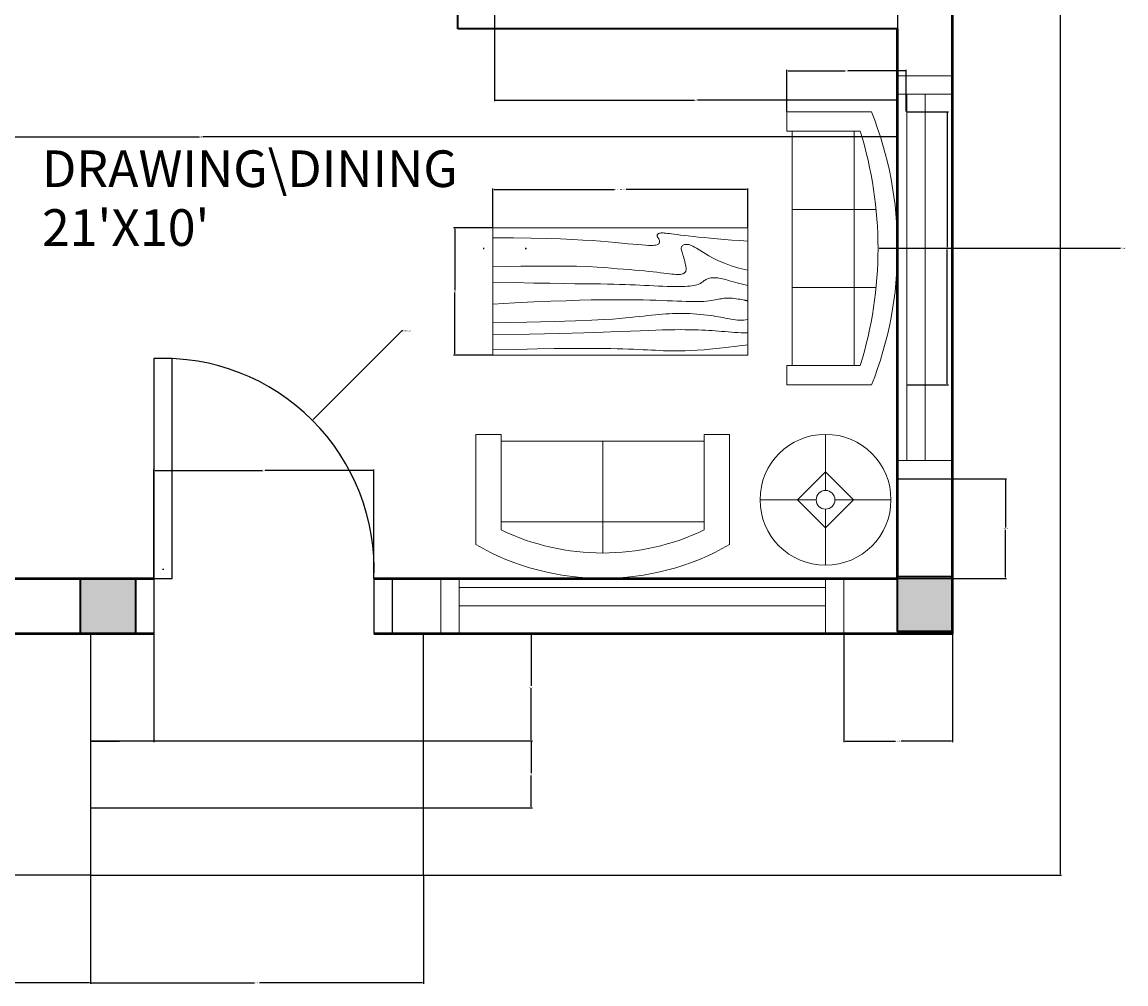
# Model space of a CAD drawing. Units: inches. Extents: x 2421 to 2780, y 382 to 769.
# Tile 2 of 4: x 2599 to 2780, y 382 to 539. Entities that reach past the tile are written whole.
import ezdxf

# ---------------------------------------------------------------- set-up
doc = ezdxf.new("R2010")
doc.units = ezdxf.units.IN
for name, color, linetype, lineweight in [('A-ANNO-DIMS', 2, 'Continuous', 18), ('A-AREA-IDEN', 7, 'Continuous', 25), ('A-COLS', 1, 'Continuous', 35), ('A-FLOR-STRS', 7, 'Continuous', 25), ('DOOR', 1, 'Continuous', 25), ('FURNITURE', 3, 'Continuous', 18), ('INNER WALL', 2, 'Continuous', 35), ('OUTER WALL', 4, 'Continuous', 50), ('WINDOW', 5, 'Continuous', 18)]:
    doc.layers.add(name, color=color, linetype=linetype, lineweight=lineweight)
doc.styles.get("Standard").update_dxf_attribs({"font": 'arial.ttf'})
doc.dimstyles.get("Standard").update_dxf_attribs({"dimtxt": 0.18, "dimasz": 0.18, "dimexe": 0.18, "dimexo": 0.0625, "dimgap": 0.09, "dimtad": 0, "dimtih": 1, "dimtoh": 1, "dimdec": 4, "dimzin": 0, "dimdsep": 46, "dimtxsty": 'Standard', "dimcen": 0.09, "dimadec": 0, "dimazin": 0, "dimtfac": 1, "dimtdec": 4, "dimtofl": 0, "dimtmove": 0, "dimatfit": 3, "dimfxl": 1, "dimtolj": 1, "dimtzin": 0, "dimarcsym": 0})

# ---------------------------------------------------------------- blocks, each defined once
blk = doc.blocks.new('Sofa - Roundback 7 ft.')
for p, q in [((-12.00002, -32.4421), (-12.00003, -6.5971)), ((11.99997, -32.4421), (11.99998, -6.5971)), ((-36.000027, -34), (-36.000027, -11.4696)), ((-35.999844, -13.3819), (35.9998, -13.3819)), ((35.99998, -34), (35.99998, -11.4696)), ((-36.000027, -32.4421), (35.99998, -32.4421))]:
    blk.add_line(p, q)
for points in [[(-36.000027, -34), (-42.000027, -34), (-42.000027, -8)], [(41.99998, -8), (41.99998, -34), (35.99998, -34)]]:
    blk.add_lwpolyline(points)
for centre, radius, start, end in [((0, -114.25), 114.25, 68.43141, 111.5686), ((-0.00001, -127.1968), 121.1968, 72.72033, 107.2797)]:
    blk.add_arc(centre, radius, start, end)
blk = doc.blocks.new('Table - Rectangular Woodgrain 60 x 30 in.')
for p, q in [((0, 0), (0, -30)), ((60, 0), (0, 0)), ((60, -30), (60, 0)), ((0, -30), (60, -30))]:
    blk.add_line(p, q)
for points in [[(0, -2.4), (4.8155, -2.418), (9.0302, -2.4688), (12.709, -2.5477), (15.9167, -2.65), (18.7181, -2.7711), (21.1781, -2.9063), (23.3616, -3.0508), (25.3333, -3.2), (27.1477, -3.3495), (28.8172, -3.4958), (30.3437, -3.636), (31.7291, -3.7667), (32.9756, -3.8849), (34.0849, -3.9875), (35.059, -4.0714), (35.9, -4.1334), (36.6114, -4.1711), (37.2041, -4.1854), (37.6906, -4.1779), (38.0833, -4.15), (38.3948, -4.1034), (38.6375, -4.0396), (38.8239, -3.9602), (38.9666, -3.8667), (39.0764, -3.7608), (39.1573, -3.6448), (39.2116, -3.521), (39.2416, -3.3917), (39.2498, -3.2593), (39.2385, -3.1261), (39.21, -2.9944), (39.1666, -2.8667), (39.111, -2.7447), (39.0468, -2.6281), (38.978, -2.5163), (38.9083, -2.4083), (38.8418, -2.3035), (38.7823, -2.201), (38.7337, -2.1001), (38.7, -2), (38.6844, -1.9003), (38.6875, -1.8021), (38.7094, -1.707), (38.75, -1.6167), (38.8094, -1.5326), (38.8875, -1.4563), (38.9844, -1.3893), (39.1, -1.3333), (39.2351, -1.2896), (39.3937, -1.2583), (39.5804, -1.2396), (39.8, -1.2333), (40.057, -1.2396), (40.3562, -1.2583), (40.7023, -1.2896), (41.1, -1.3333), (41.5547, -1.3895), (42.0755, -1.4573), (42.6721, -1.5361), (43.3542, -1.625), (44.1316, -1.7233), (45.014, -1.8302), (46.0114, -1.9449), (47.1333, -2.0667), (48.3862, -2.1947), (49.7625, -2.3281), (51.2513, -2.4663), (52.8416, -2.6083), (54.5226, -2.7535), (56.2833, -2.9011), (58.1127, -3.0501), (60, -3.2)], [(0, -9.2), (6.5759, -9.0858), (11.9385, -9.0365), (16.2527, -9.0418), (19.6833, -9.0917), (22.3952, -9.1759), (24.5531, -9.2844), (26.322, -9.4069), (27.8666, -9.5333), (29.3241, -9.6553), (30.7203, -9.7719), (32.0532, -9.8837), (33.3208, -9.9917), (34.5213, -10.0965), (35.6526, -10.199), (36.7128, -10.2999), (37.7, -10.4), (38.6129, -10.4996), (39.4531, -10.5969), (40.223, -10.6895), (40.925, -10.775), (41.5613, -10.8512), (42.1344, -10.9156), (42.6465, -10.966), (43.1, -11), (43.4976, -11.0158), (43.8437, -11.0136), (44.143, -10.9942), (44.4, -10.9583), (44.6195, -10.9069), (44.8062, -10.8406), (44.9648, -10.7603), (45.1, -10.6667), (45.2155, -10.5598), (45.3114, -10.4365), (45.3871, -10.2929), (45.4416, -10.125), (45.4743, -9.929), (45.4844, -9.7011), (45.4709, -9.4371), (45.4333, -9.1333), (45.3716, -8.7883), (45.2896, -8.4104), (45.1919, -8.0107), (45.0833, -7.6), (44.9685, -7.1893), (44.8521, -6.7896), (44.7388, -6.4117), (44.6333, -6.0667), (44.54, -5.7628), (44.4614, -5.4979), (44.4001, -5.2675), (44.3583, -5.0667), (44.3384, -4.8909), (44.3427, -4.7354), (44.3736, -4.5956), (44.4333, -4.4667), (44.5236, -4.3453), (44.6427, -4.2333), (44.7884, -4.1339), (44.9583, -4.05), (45.1501, -3.9849), (45.3614, -3.9417), (45.59, -3.9234), (45.8333, -3.9333), (46.0915, -3.9749), (46.3734, -4.0531), (46.6906, -4.1736), (47.0542, -4.3417), (47.4756, -4.5629), (47.9661, -4.8427), (48.5372, -5.1866), (49.2, -5.6), (49.9676, -6.0844), (50.8594, -6.625), (51.8965, -7.2031), (53.1, -7.8), (54.491, -8.3969), (56.0906, -8.975), (57.9199, -9.5156), (60, -10)], [(0, -12.8), (5.1847, -12.9322), (9.6213, -13.0323), (13.3963, -13.1059), (16.5958, -13.1583), (19.3063, -13.1952), (21.614, -13.2219), (23.6054, -13.2439), (25.3666, -13.2667), (26.9728, -13.2947), (28.4531, -13.3281), (29.8256, -13.3663), (31.1083, -13.4083), (32.3191, -13.4535), (33.476, -13.501), (34.597, -13.5501), (35.7, -13.6), (36.7984, -13.6497), (37.8875, -13.6979), (38.9578, -13.743), (40, -13.7833), (41.0047, -13.8174), (41.9625, -13.8438), (42.864, -13.8607), (43.7, -13.8667), (44.4631, -13.8604), (45.1552, -13.8417), (45.7801, -13.8104), (46.3416, -13.7667), (46.8439, -13.7104), (47.2906, -13.6417), (47.6858, -13.5604), (48.0333, -13.4667), (48.3375, -13.3608), (48.6042, -13.2448), (48.8396, -13.121), (49.05, -12.9917), (49.2417, -12.8593), (49.4208, -12.7261), (49.5937, -12.5944), (49.7667, -12.4667), (49.9452, -12.3451), (50.1323, -12.2313), (50.3303, -12.1268), (50.5416, -12.0333), (50.7686, -11.9524), (51.0135, -11.8854), (51.2788, -11.8341), (51.5666, -11.8), (51.8785, -11.7843), (52.2116, -11.7865), (52.562, -11.8059), (52.926, -11.8417), (53.2998, -11.8931), (53.6795, -11.9594), (54.0614, -12.0397), (54.4416, -12.1333), (54.8223, -12.2401), (55.2293, -12.3625), (55.6942, -12.5037), (56.2489, -12.6667), (56.9251, -12.8547), (57.7545, -13.0708), (58.7689, -13.3182), (60, -13.6)], [(0, -18), (5.124, -17.7273), (9.6609, -17.5057), (13.6705, -17.3303), (17.2125, -17.1958), (20.3467, -17.0973), (23.1328, -17.0297), (25.6307, -16.9878), (27.9, -16.9667), (29.9928, -16.9617), (31.9302, -16.9703), (33.7254, -16.9907), (35.3917, -17.0208), (36.9423, -17.0588), (38.3906, -17.1026), (39.7499, -17.1503), (41.0333, -17.2), (42.2519, -17.2496), (43.4073, -17.2969), (44.4986, -17.3395), (45.525, -17.375), (46.4858, -17.4012), (47.3802, -17.4156), (48.2074, -17.416), (48.9667, -17.4), (49.6583, -17.3662), (50.2872, -17.3167), (50.8595, -17.2547), (51.3812, -17.1833), (51.8584, -17.1057), (52.2971, -17.025), (52.7034, -16.9443), (53.0833, -16.8667), (53.443, -16.7951), (53.789, -16.7313), (54.128, -16.6768), (54.4666, -16.6334), (54.8115, -16.6024), (55.1693, -16.5854), (55.5465, -16.5841), (55.95, -16.6), (56.3828, -16.6337), (56.8346, -16.6823), (57.2915, -16.7418), (57.7396, -16.8084), (58.165, -16.878), (58.5539, -16.9469), (58.8924, -17.0111), (59.1666, -17.0667), (59.3679, -17.1107), (59.5078, -17.1438), (59.6032, -17.1675), (59.6708, -17.1833), (59.7275, -17.193), (59.7901, -17.1979), (59.8753, -17.1998), (60, -17.2)], [(0, -22.4), (8.0098, -22.2501), (14.4094, -22.1011), (19.4168, -21.9535), (23.25, -21.8083), (26.1269, -21.6663), (28.2656, -21.5281), (29.884, -21.3947), (31.2, -21.2667), (32.3967, -21.1448), (33.5172, -21.0292), (34.5697, -20.9198), (35.5625, -20.8167), (36.5037, -20.7198), (37.4015, -20.6292), (38.2642, -20.5448), (39.1, -20.4667), (39.9164, -20.3951), (40.7187, -20.3313), (41.5117, -20.2768), (42.3, -20.2333), (43.0883, -20.2024), (43.8812, -20.1854), (44.6836, -20.1841), (45.5, -20.2), (46.3328, -20.234), (47.1747, -20.2844), (48.0163, -20.3488), (48.8479, -20.425), (49.66, -20.5106), (50.4429, -20.6031), (51.1872, -20.7004), (51.8833, -20.8), (52.5246, -20.8999), (53.1166, -20.9995), (53.6681, -21.0983), (54.1875, -21.1958), (54.6834, -21.2919), (55.1646, -21.3859), (55.6394, -21.4777), (56.1167, -21.5667), (56.6028, -21.6515), (57.0961, -21.7266), (57.5929, -21.7852), (58.0896, -21.8208), (58.5823, -21.8268), (59.0674, -21.7964), (59.5412, -21.723), (60, -21.6)], [(0, -25.2), (8.6355, -25.0504), (15.7026, -24.9031), (21.4049, -24.7606), (25.9458, -24.625), (29.529, -24.4988), (32.3578, -24.3844), (34.6359, -24.284), (36.5667, -24.2), (38.3213, -24.1341), (39.9417, -24.0854), (41.437, -24.0523), (42.8167, -24.0333), (44.0901, -24.0268), (45.2667, -24.0313), (46.3557, -24.0451), (47.3667, -24.0667), (48.309, -24.0947), (49.1928, -24.1287), (50.0284, -24.168), (50.826, -24.2125), (51.5959, -24.2617), (52.3483, -24.3151), (53.0935, -24.3725), (53.8417, -24.4334), (54.6009, -24.497), (55.3699, -24.561), (56.1454, -24.6226), (56.9239, -24.6792), (57.7021, -24.7279), (58.4764, -24.7662), (59.2435, -24.7911), (60, -24.8)], [(0, -28.8), (5.6867, -28.6681), (10.45, -28.5698), (14.407, -28.5012), (17.675, -28.4584), (20.3711, -28.4374), (22.6125, -28.4344), (24.5164, -28.4455), (26.2, -28.4667), (27.762, -28.4947), (29.2276, -28.5281), (30.6033, -28.5663), (31.8958, -28.6084), (33.1118, -28.6535), (34.2578, -28.7011), (35.3405, -28.7501), (36.3666, -28.8), (37.3443, -28.8497), (38.288, -28.8974), (39.2137, -28.9412), (40.1375, -28.9792), (41.0753, -29.0093), (42.0432, -29.0297), (43.0572, -29.0384), (44.1333, -29.0333), (45.2936, -29.0114), (46.5843, -28.9641), (48.0579, -28.8816), (49.7666, -28.7542), (51.7629, -28.5721), (54.0989, -28.3255), (56.8272, -28.0048), (60, -27.6)]]:
    blk.add_lwpolyline(points)
blk = doc.blocks.new('Lamp - Table')
for p, q in [((0, 7), (0, 1)), ((0, 3), (-3, 0)), ((3, 0), (0, 3)), ((-1, 0), (-7, 0)), ((-3, 0), (0, -3)), ((0, -3), (3, 0)), ((1, 0), (7, 0)), ((0, -1), (0, -7))]:
    blk.add_line(p, q)
for radius in [7, 1]:
    blk.add_circle((0, 0), radius)
blk = doc.blocks.new('Sofa - Roundback Loveseat 5 ft.')
for p, q in [((0, -32.44198), (0, -5.99998)), ((-24, -33.99998), (-24, -11.46958)), ((24.00004, -33.99998), (24.00004, -11.46958)), ((-23.9998, -13.38178), (23.99986, -13.38178)), ((-24, -32.44198), (24.00004, -32.44198))]:
    blk.add_line(p, q)
for points in [[(-24, -33.99998), (-30, -33.99998), (-30, -7.99998)], [(30.00004, -7.99998), (30.00004, -33.99998), (24.00004, -33.99998)]]:
    blk.add_lwpolyline(points)
for centre, radius, start, end in [((0, -60.24998), 60.24998, 60.13715, 119.8628), ((0, -61.38438), 55.38444, 64.32083, 115.6792)]:
    blk.add_arc(centre, radius, start, end)
blk = doc.blocks.new('WIN-60IN')
for p, q in [((0, 0), (0, 9)), ((3, 0), (3, 9)), ((63, 9), (63, 0)), ((66, 9), (66, 0)), ((63, 4.5), (3, 4.5)), ((63, 1.5), (3, 1.5))]:
    blk.add_line(p, q)
blk = doc.blocks.new('COL-9X9IN')
h = blk.add_hatch(color=256)
h.dxf.hatch_style = 1
h.paths.add_polyline_path([(9, 9), (0, 9), (0, 0), (9, 0)])
blk.add_lwpolyline([(0, 9), (9, 9), (9, 0), (0, 0)], close=True)
blk = doc.blocks.new('*D38')
at = {"layer": 'A-ANNO-DIMS', "color": 0, "lineweight": -2, "transparency": 16777216}
for p, q in [((2743.95, 524.61), (2750.78, 524.61)), ((2750.6, 524.43), (2750.6, 502.42)), ((2750.6, 480.04), (2750.6, 502.05)), ((2743.95, 479.86), (2750.78, 479.86))]:
    blk.add_line(p, q, dxfattribs=at)
at = {"layer": 'A-ANNO-DIMS', "color": 0, "transparency": 16777216}
for points in [[(2750.57, 524.43), (2750.63, 524.43), (2750.6, 524.61)], [(2750.57, 480.04), (2750.63, 480.04), (2750.6, 479.86)]]:
    blk.add_solid(points, dxfattribs=at)
at = {"layer": 'Defpoints', "color": 0, "transparency": 16777216}
for p in [(2743.89, 524.61), (2743.89, 479.86), (2750.6, 479.86)]:
    blk.add_point(p, dxfattribs=at)
at = {"layer": 'A-ANNO-DIMS', "color": 0, "transparency": 16777216, "insert": (2750.6, 502.23), "char_height": 0.18, "attachment_point": 5}
blk.add_mtext('\\A1;SOFA 45', dxfattribs=at)
blk = doc.blocks.new('*D39')
at = {"layer": 'A-ANNO-DIMS', "color": 0, "lineweight": -2, "transparency": 16777216}
for p, q in [((2724.35, 524.67), (2724.35, 531.5)), ((2724.53, 531.32), (2733.9, 531.32)), ((2743.71, 531.32), (2734.34, 531.32)), ((2743.89, 524.67), (2743.89, 531.5))]:
    blk.add_line(p, q, dxfattribs=at)
at = {"layer": 'A-ANNO-DIMS', "color": 0, "transparency": 16777216}
for points in [[(2724.53, 531.35), (2724.53, 531.29), (2724.35, 531.32)], [(2743.71, 531.35), (2743.71, 531.29), (2743.89, 531.32)]]:
    blk.add_solid(points, dxfattribs=at)
at = {"layer": 'Defpoints', "color": 0, "transparency": 16777216}
for p in [(2743.89, 531.32), (2724.35, 524.61), (2743.89, 524.61)]:
    blk.add_point(p, dxfattribs=at)
at = {"layer": 'A-ANNO-DIMS', "color": 0, "transparency": 16777216, "insert": (2734.12, 531.32), "char_height": 0.18, "attachment_point": 5}
blk.add_mtext('\\A1;20', dxfattribs=at)
blk = doc.blocks.new('*D40')
at = {"layer": 'A-ANNO-DIMS', "color": 0, "lineweight": -2, "transparency": 16777216}
for p, q in [((2676.23, 505.69), (2676.23, 512.06)), ((2676.41, 511.88), (2696.11, 511.88)), ((2717.76, 511.88), (2698.05, 511.88)), ((2717.94, 505.69), (2717.94, 512.06))]:
    blk.add_line(p, q, dxfattribs=at)
at = {"layer": 'A-ANNO-DIMS', "color": 0, "transparency": 16777216}
for points in [[(2676.41, 511.91), (2676.41, 511.85), (2676.23, 511.88)], [(2717.76, 511.91), (2717.76, 511.85), (2717.94, 511.88)]]:
    blk.add_solid(points, dxfattribs=at)
at = {"layer": 'Defpoints', "color": 0, "transparency": 16777216}
for p in [(2717.94, 511.88), (2676.23, 505.62), (2717.94, 505.62)]:
    blk.add_point(p, dxfattribs=at)
at = {"layer": 'A-ANNO-DIMS', "color": 0, "transparency": 16777216, "insert": (2697.08, 511.88), "char_height": 0.18, "attachment_point": 5}
blk.add_mtext('\\A1;LOW TABLE 42', dxfattribs=at)
blk = doc.blocks.new('*D41')
at = {"layer": 'A-ANNO-DIMS', "color": 0, "lineweight": -2, "transparency": 16777216}
for p, q in [((2676.17, 505.62), (2669.79, 505.62)), ((2669.97, 505.44), (2669.97, 495.38)), ((2669.97, 484.95), (2669.97, 495.02)), ((2676.17, 484.77), (2669.79, 484.77))]:
    blk.add_line(p, q, dxfattribs=at)
at = {"layer": 'A-ANNO-DIMS', "color": 0, "transparency": 16777216}
for points in [[(2669.94, 505.44), (2670, 505.44), (2669.97, 505.62)], [(2669.94, 484.95), (2670, 484.95), (2669.97, 484.77)]]:
    blk.add_solid(points, dxfattribs=at)
at = {"layer": 'Defpoints', "color": 0, "transparency": 16777216}
for p in [(2669.97, 505.62), (2676.23, 505.62), (2676.23, 484.77)]:
    blk.add_point(p, dxfattribs=at)
at = {"layer": 'A-ANNO-DIMS', "color": 0, "transparency": 16777216, "insert": (2669.97, 495.2), "char_height": 0.18, "attachment_point": 5}
blk.add_mtext('\\A1;21', dxfattribs=at)
blk = doc.blocks.new('*D47')
at = {"layer": 'A-ANNO-DIMS', "color": 0, "lineweight": -2, "transparency": 16777216}
for p, q in [((2751.53, 751.18), (2769.3, 751.18)), ((2769.12, 751), (2769.12, 575.56)), ((2769.12, 399.76), (2769.12, 575.2)), ((2664.93, 399.58), (2769.3, 399.58))]:
    blk.add_line(p, q, dxfattribs=at)
at = {"layer": 'A-ANNO-DIMS', "color": 0, "transparency": 16777216}
for points in [[(2769.09, 751), (2769.15, 751), (2769.12, 751.18)], [(2769.09, 399.76), (2769.15, 399.76), (2769.12, 399.58)]]:
    blk.add_solid(points, dxfattribs=at)
at = {"layer": 'Defpoints', "color": 0, "transparency": 16777216}
for p in [(2751.47, 751.18), (2664.86, 399.58), (2769.12, 399.58)]:
    blk.add_point(p, dxfattribs=at)
at = {"layer": 'A-ANNO-DIMS', "color": 0, "transparency": 16777216, "insert": (2769.12, 575.38), "char_height": 0.18, "attachment_point": 5}
blk.add_mtext('\\A1;351.6', dxfattribs=at)
blk = doc.blocks.new('*D48')
at = {"layer": 'A-ANNO-DIMS', "color": 0, "lineweight": -2, "transparency": 16777216}
for p, q in [((2610.35, 399.52), (2610.35, 381.75)), ((2664.86, 399.52), (2664.86, 381.75)), ((2610.53, 381.93), (2637.21, 381.93)), ((2664.68, 381.93), (2638, 381.93))]:
    blk.add_line(p, q, dxfattribs=at)
at = {"layer": 'A-ANNO-DIMS', "color": 0, "transparency": 16777216}
for points in [[(2610.53, 381.96), (2610.53, 381.9), (2610.35, 381.93)], [(2664.68, 381.96), (2664.68, 381.9), (2664.86, 381.93)]]:
    blk.add_solid(points, dxfattribs=at)
at = {"layer": 'Defpoints', "color": 0, "transparency": 16777216}
for p in [(2610.35, 399.58), (2664.86, 399.58), (2664.86, 381.93)]:
    blk.add_point(p, dxfattribs=at)
at = {"layer": 'A-ANNO-DIMS', "color": 0, "transparency": 16777216, "insert": (2637.61, 381.93), "char_height": 0.18, "attachment_point": 5}
blk.add_mtext('\\A1;54.52', dxfattribs=at)
blk = doc.blocks.new('*D49')
at = {"layer": 'A-ANNO-DIMS', "color": 0, "lineweight": -2, "transparency": 16777216}
for p, q in [((2439.47, 439.12), (2439.47, 381.75)), ((2610.35, 439.12), (2610.35, 381.75)), ((2439.65, 381.93), (2524.45, 381.93)), ((2610.17, 381.93), (2525.36, 381.93))]:
    blk.add_line(p, q, dxfattribs=at)
at = {"layer": 'A-ANNO-DIMS', "color": 0, "transparency": 16777216}
for points in [[(2439.65, 381.96), (2439.65, 381.9), (2439.47, 381.93)], [(2610.17, 381.96), (2610.17, 381.9), (2610.35, 381.93)]]:
    blk.add_solid(points, dxfattribs=at)
at = {"layer": 'Defpoints', "color": 0, "transparency": 16777216}
for p in [(2439.47, 439.18), (2610.35, 439.18), (2610.35, 381.93)]:
    blk.add_point(p, dxfattribs=at)
at = {"layer": 'A-ANNO-DIMS', "color": 0, "transparency": 16777216, "insert": (2524.91, 381.93), "char_height": 0.18, "attachment_point": 5}
blk.add_mtext('\\A1;170.88', dxfattribs=at)
blk = doc.blocks.new('*D50')
at = {"layer": 'A-ANNO-DIMS', "color": 0, "lineweight": -2, "transparency": 16777216}
for p, q in [((2439.4, 439.18), (2421.64, 439.18)), ((2421.82, 439), (2421.82, 419.56)), ((2421.82, 399.76), (2421.82, 419.2)), ((2610.28, 399.58), (2421.64, 399.58))]:
    blk.add_line(p, q, dxfattribs=at)
at = {"layer": 'A-ANNO-DIMS', "color": 0, "transparency": 16777216}
for points in [[(2421.79, 439), (2421.85, 439), (2421.82, 439.18)], [(2421.79, 399.76), (2421.85, 399.76), (2421.82, 399.58)]]:
    blk.add_solid(points, dxfattribs=at)
at = {"layer": 'Defpoints', "color": 0, "transparency": 16777216}
for p in [(2421.82, 439.18), (2439.47, 439.18), (2610.35, 399.58)]:
    blk.add_point(p, dxfattribs=at)
at = {"layer": 'A-ANNO-DIMS', "color": 0, "transparency": 16777216, "insert": (2421.82, 419.38), "char_height": 0.18, "attachment_point": 5}
blk.add_mtext('\\A1;39.6', dxfattribs=at)
blk = doc.blocks.new('*D53')
at = {"layer": 'A-ANNO-DIMS', "color": 0, "lineweight": -2, "transparency": 16777216}
for p, q in [((2676.47, 544.12), (2676.47, 526.35)), ((2742.47, 544.12), (2742.47, 526.35)), ((2676.65, 526.53), (2709.25, 526.53)), ((2742.29, 526.53), (2709.69, 526.53))]:
    blk.add_line(p, q, dxfattribs=at)
at = {"layer": 'A-ANNO-DIMS', "color": 0, "transparency": 16777216}
for points in [[(2676.65, 526.56), (2676.65, 526.5), (2676.47, 526.53)], [(2742.29, 526.56), (2742.29, 526.5), (2742.47, 526.53)]]:
    blk.add_solid(points, dxfattribs=at)
at = {"layer": 'Defpoints', "color": 0, "transparency": 16777216}
for p in [(2676.47, 544.18), (2742.47, 544.18), (2676.47, 526.53)]:
    blk.add_point(p, dxfattribs=at)
at = {"layer": 'A-ANNO-DIMS', "color": 0, "transparency": 16777216, "insert": (2709.47, 526.53), "char_height": 0.18, "attachment_point": 5}
blk.add_mtext('\\A1;66', dxfattribs=at)
blk = doc.blocks.new('*D54')
at = {"layer": 'A-ANNO-DIMS', "color": 0, "lineweight": -2, "transparency": 16777216}
for p, q in [((2514.47, 538.12), (2514.47, 520.35)), ((2742.47, 538.12), (2742.47, 520.35)), ((2514.65, 520.53), (2628.18, 520.53)), ((2742.29, 520.53), (2628.76, 520.53))]:
    blk.add_line(p, q, dxfattribs=at)
at = {"layer": 'A-ANNO-DIMS', "color": 0, "transparency": 16777216}
for points in [[(2514.65, 520.56), (2514.65, 520.5), (2514.47, 520.53)], [(2742.29, 520.56), (2742.29, 520.5), (2742.47, 520.53)]]:
    blk.add_solid(points, dxfattribs=at)
at = {"layer": 'Defpoints', "color": 0, "transparency": 16777216}
for p in [(2514.47, 538.18), (2742.47, 538.18), (2514.47, 520.53)]:
    blk.add_point(p, dxfattribs=at)
at = {"layer": 'A-ANNO-DIMS', "color": 0, "transparency": 16777216, "insert": (2628.47, 520.53), "char_height": 0.18, "attachment_point": 5}
blk.add_mtext('\\A1;228', dxfattribs=at)
blk = doc.blocks.new('*D63')
at = {"layer": 'A-ANNO-DIMS', "color": 0, "lineweight": -2, "transparency": 16777216}
for p, q in [((2742.53, 464.51), (2760.3, 464.51)), ((2760.12, 464.33), (2760.12, 456.53)), ((2760.12, 448.36), (2760.12, 456.16)), ((2742.53, 448.18), (2760.3, 448.18))]:
    blk.add_line(p, q, dxfattribs=at)
at = {"layer": 'A-ANNO-DIMS', "color": 0, "transparency": 16777216}
for points in [[(2760.09, 464.33), (2760.15, 464.33), (2760.12, 464.51)], [(2760.09, 448.36), (2760.15, 448.36), (2760.12, 448.18)]]:
    blk.add_solid(points, dxfattribs=at)
at = {"layer": 'Defpoints', "color": 0, "transparency": 16777216}
for p in [(2742.47, 464.51), (2742.47, 448.18), (2760.12, 448.18)]:
    blk.add_point(p, dxfattribs=at)
at = {"layer": 'A-ANNO-DIMS', "color": 0, "transparency": 16777216, "insert": (2760.12, 456.34), "char_height": 0.18, "attachment_point": 5}
blk.add_mtext('\\A1;16.328', dxfattribs=at)
blk = doc.blocks.new('*D65')
at = {"layer": 'A-ANNO-DIMS', "color": 0, "lineweight": -2, "transparency": 16777216}
for p, q in [((2610.35, 439.12), (2610.35, 421.35)), ((2620.74, 439.12), (2620.74, 421.35)), ((2610.53, 421.53), (2615.1, 421.53)), ((2620.56, 421.53), (2615.98, 421.53))]:
    blk.add_line(p, q, dxfattribs=at)
at = {"layer": 'A-ANNO-DIMS', "color": 0, "transparency": 16777216}
for points in [[(2610.53, 421.56), (2610.53, 421.5), (2610.35, 421.53)], [(2620.56, 421.56), (2620.56, 421.5), (2620.74, 421.53)]]:
    blk.add_solid(points, dxfattribs=at)
at = {"layer": 'Defpoints', "color": 0, "transparency": 16777216}
for p in [(2610.35, 439.18), (2620.74, 439.18), (2610.35, 421.53)]:
    blk.add_point(p, dxfattribs=at)
at = {"layer": 'A-ANNO-DIMS', "color": 0, "transparency": 16777216, "insert": (2615.54, 421.53), "char_height": 0.18, "attachment_point": 5}
blk.add_mtext('\\A1;10.391', dxfattribs=at)
blk = doc.blocks.new('*D66')
at = {"layer": 'A-ANNO-DIMS', "color": 0, "lineweight": -2, "transparency": 16777216}
for p, q in [((2620.74, 448.24), (2620.74, 466.01)), ((2620.92, 465.83), (2638.52, 465.83)), ((2656.56, 465.83), (2638.96, 465.83)), ((2656.74, 448.24), (2656.74, 466.01))]:
    blk.add_line(p, q, dxfattribs=at)
at = {"layer": 'A-ANNO-DIMS', "color": 0, "transparency": 16777216}
for points in [[(2620.92, 465.86), (2620.92, 465.8), (2620.74, 465.83)], [(2656.56, 465.86), (2656.56, 465.8), (2656.74, 465.83)]]:
    blk.add_solid(points, dxfattribs=at)
at = {"layer": 'Defpoints', "color": 0, "transparency": 16777216}
for p in [(2656.74, 465.83), (2620.74, 448.18), (2656.74, 448.18)]:
    blk.add_point(p, dxfattribs=at)
at = {"layer": 'A-ANNO-DIMS', "color": 0, "transparency": 16777216, "insert": (2638.74, 465.83), "char_height": 0.18, "attachment_point": 5}
blk.add_mtext('\\A1;36', dxfattribs=at)
blk = doc.blocks.new('*D67')
at = {"layer": 'A-ANNO-DIMS', "color": 0, "lineweight": -2, "transparency": 16777216}
for p, q in [((2733.68, 439.12), (2733.68, 421.35)), ((2751.47, 439.12), (2751.47, 421.35)), ((2733.86, 421.53), (2742.12, 421.53)), ((2751.29, 421.53), (2743.03, 421.53))]:
    blk.add_line(p, q, dxfattribs=at)
at = {"layer": 'A-ANNO-DIMS', "color": 0, "transparency": 16777216}
for points in [[(2733.86, 421.56), (2733.86, 421.5), (2733.68, 421.53)], [(2751.29, 421.56), (2751.29, 421.5), (2751.47, 421.53)]]:
    blk.add_solid(points, dxfattribs=at)
at = {"layer": 'Defpoints', "color": 0, "transparency": 16777216}
for p in [(2733.68, 439.18), (2751.47, 439.18), (2733.68, 421.53)]:
    blk.add_point(p, dxfattribs=at)
at = {"layer": 'A-ANNO-DIMS', "color": 0, "transparency": 16777216, "insert": (2742.57, 421.53), "char_height": 0.18, "attachment_point": 5}
blk.add_mtext('\\A1;17.785', dxfattribs=at)
blk = doc.blocks.new('*D72')
at = {"layer": 'A-ANNO-DIMS', "color": 0, "lineweight": -2, "transparency": 16777216}
for p, q in [((2664.93, 439.18), (2682.69, 439.18)), ((2682.51, 439), (2682.51, 430.56)), ((2682.51, 421.76), (2682.51, 430.2)), ((2664.93, 421.58), (2682.69, 421.58))]:
    blk.add_line(p, q, dxfattribs=at)
at = {"layer": 'A-ANNO-DIMS', "color": 0, "transparency": 16777216}
for points in [[(2682.48, 439), (2682.54, 439), (2682.51, 439.18)], [(2682.48, 421.76), (2682.54, 421.76), (2682.51, 421.58)]]:
    blk.add_solid(points, dxfattribs=at)
at = {"layer": 'Defpoints', "color": 0, "transparency": 16777216}
for p in [(2664.86, 439.18), (2664.86, 421.58), (2682.51, 421.58)]:
    blk.add_point(p, dxfattribs=at)
at = {"layer": 'A-ANNO-DIMS', "color": 0, "transparency": 16777216, "insert": (2682.51, 430.38), "char_height": 0.18, "attachment_point": 5}
blk.add_mtext('\\A1;17.598', dxfattribs=at)
blk = doc.blocks.new('*D73')
at = {"layer": 'A-ANNO-DIMS', "color": 0, "lineweight": -2, "transparency": 16777216}
for p, q in [((2664.93, 421.58), (2682.69, 421.58)), ((2682.51, 421.4), (2682.51, 416.26)), ((2682.51, 410.76), (2682.51, 415.9)), ((2664.93, 410.58), (2682.69, 410.58))]:
    blk.add_line(p, q, dxfattribs=at)
at = {"layer": 'A-ANNO-DIMS', "color": 0, "transparency": 16777216}
for points in [[(2682.48, 421.4), (2682.54, 421.4), (2682.51, 421.58)], [(2682.48, 410.76), (2682.54, 410.76), (2682.51, 410.58)]]:
    blk.add_solid(points, dxfattribs=at)
at = {"layer": 'Defpoints', "color": 0, "transparency": 16777216}
for p in [(2664.86, 421.58), (2664.86, 410.58), (2682.51, 410.58)]:
    blk.add_point(p, dxfattribs=at)
at = {"layer": 'A-ANNO-DIMS', "color": 0, "transparency": 16777216, "insert": (2682.51, 416.08), "char_height": 0.18, "attachment_point": 5}
blk.add_mtext('\\A1;11', dxfattribs=at)
blk = doc.blocks.new('*D74')
at = {"layer": 'A-ANNO-DIMS', "color": 0, "lineweight": -2, "transparency": 16777216}
for p, q in [((2661.31, 488.75), (2646.78, 474.23)), ((2661.49, 488.75), (2661.31, 488.75)), ((2622.15, 449.68), (2622.33, 449.68)), ((2622.24, 449.59), (2622.24, 449.77))]:
    blk.add_line(p, q, dxfattribs=at)
at = {"layer": 'A-ANNO-DIMS', "color": 0, "transparency": 16777216}
blk.add_solid([(2646.76, 474.25), (2646.8, 474.21), (2646.66, 474.1)], dxfattribs=at)
at = {"layer": 'Defpoints', "color": 0, "transparency": 16777216}
for p in [(2646.66, 474.1), (2622.24, 449.68)]:
    blk.add_point(p, dxfattribs=at)
at = {"layer": 'A-ANNO-DIMS', "color": 0, "transparency": 16777216, "insert": (2662.16, 488.75), "char_height": 0.18, "attachment_point": 5}
blk.add_mtext('\\A1;5X R34.53', dxfattribs=at)
blk = doc.blocks.new('*D75')
at = {"layer": 'A-ANNO-DIMS', "color": 0, "lineweight": -2, "transparency": 16777216}
for p, q in [((2674.62, 502.23), (2674.8, 502.23)), ((2674.71, 502.14), (2674.71, 502.32)), ((2778.01, 502.24), (2739.45, 502.24))]:
    blk.add_line(p, q, dxfattribs=at)
at = {"layer": 'A-ANNO-DIMS', "color": 0, "transparency": 16777216}
blk.add_solid([(2739.45, 502.27), (2739.45, 502.21), (2739.27, 502.24)], dxfattribs=at)
at = {"layer": 'Defpoints', "color": 0, "transparency": 16777216}
for p in [(2674.71, 502.23), (2739.27, 502.24)]:
    blk.add_point(p, dxfattribs=at)
at = {"layer": 'A-ANNO-DIMS', "color": 0, "transparency": 16777216, "insert": (2778.49, 502.24), "char_height": 0.18, "attachment_point": 5}
blk.add_mtext('\\A1;R64.56', dxfattribs=at)
blk = doc.blocks.new('*D76')
at = {"layer": 'A-ANNO-DIMS', "color": 0, "lineweight": -2, "transparency": 16777216}
for p, q in [((2681.52, 502.23), (2681.7, 502.23)), ((2681.61, 502.14), (2681.61, 502.32)), ((2778.98, 502.24), (2742.65, 502.24))]:
    blk.add_line(p, q, dxfattribs=at)
at = {"layer": 'A-ANNO-DIMS', "color": 0, "transparency": 16777216}
blk.add_solid([(2742.65, 502.27), (2742.65, 502.21), (2742.47, 502.24)], dxfattribs=at)
at = {"layer": 'Defpoints', "color": 0, "transparency": 16777216}
for p in [(2681.61, 502.23), (2742.47, 502.24)]:
    blk.add_point(p, dxfattribs=at)
at = {"layer": 'A-ANNO-DIMS', "color": 0, "transparency": 16777216, "insert": (2779.46, 502.24), "char_height": 0.18, "attachment_point": 5}
blk.add_mtext('\\A1;R60.86', dxfattribs=at)

msp = doc.modelspace()

# ---------------------------------------------------------------- linework, layer by layer
at = {"layer": 'A-FLOR-STRS'}
for p, q in [((2610.347, 439.1806), (2610.347, 399.5831)), ((2664.8646, 399.5831), (2664.8646, 439.1806)), ((2610.347, 421.5831), (2664.8646, 421.5831)), ((2610.347, 410.5831), (2664.8646, 410.5831)), ((2610.347, 399.5831), (2664.8646, 399.5831))]:
    msp.add_line(p, q, dxfattribs=at)
at = {"layer": 'DOOR'}
for p, q in [((2617.7381, 448.1806), (2617.7381, 439.1806)), ((2620.7381, 448.1806), (2620.7381, 439.1806)), ((2656.7381, 448.1806), (2656.7381, 439.1806)), ((2659.7381, 448.1806), (2659.7381, 439.1806))]:
    msp.add_line(p, q, dxfattribs=at)
msp.add_lwpolyline([(2620.7381, 448.1806), (2623.7381, 448.1806), (2623.7381, 484.1806), (2620.7381, 484.1806)], close=True, dxfattribs=at)
msp.add_arc((2622.2381, 449.6806), 34.5326, 357.510447, 92.489553, dxfattribs=at)
at = {"layer": 'INNER WALL'}
for p, q in [((2670.466, 538.1806), (2670.466, 550.1806)), ((2742.466, 538.1806), (2670.466, 538.1806))]:
    msp.add_line(p, q, dxfattribs=at)
at = {"layer": 'OUTER WALL'}
for p, q in [((2742.466, 448.1806), (2742.466, 538.1806)), ((2514.466, 448.1806), (2620.7381, 448.1806)), ((2656.7381, 448.1806), (2742.466, 448.1806))]:
    msp.add_line(p, q, dxfattribs=at)
msp.add_lwpolyline([(2656.7381, 439.1806), (2751.466, 439.1806), (2751.466, 751.1806), (2439.466, 751.1806), (2439.466, 439.1806), (2620.7381, 439.1806)], dxfattribs=at)

# ---------------------------------------------------------------- block references
at = {"layer": 'A-COLS'}
for p in [(2608.7381, 439.1806), (2742.466, 439.4812)]:
    msp.add_blockref('COL-9X9IN', p, dxfattribs=at)
at = {"layer": 'FURNITURE'}
for name, p, xscale, yscale, zscale, rotation in [('Sofa - Roundback 7 ft.', (2742.466, 502.2348), 0.532696598649806, 0.532696598649806, 0.532696598649806, 270), ('Sofa - Roundback Loveseat 5 ft.', (2694.1908, 448.1806), 0.6927207335329854, 0.6927207335329854, 0.6927207335329854, 180.0000000000006)]:
    msp.add_blockref(name, p, dxfattribs=dict(at, xscale=xscale, yscale=yscale, zscale=zscale, rotation=rotation))
for name, p, xscale, yscale, zscale in [('Table - Rectangular Woodgrain 60 x 30 in.', (2676.229, 505.6226), 0.6951231637119049, 0.6951231637119049, 0.6951231637119049), ('Lamp - Table', (2730.6695, 461.0558), 1.531444562550245, 1.531444562550245, 1.531444562550245)]:
    msp.add_blockref(name, p, dxfattribs=dict(at, xscale=xscale, yscale=yscale, zscale=zscale))
at = {"layer": 'WINDOW'}
for p, rotation in [((2742.466, 530.5086), 269.9999999999998), ((2733.6812, 448.1806), 180)]:
    msp.add_blockref('WIN-60IN', p, dxfattribs=dict(at, rotation=rotation))

# ---------------------------------------------------------------- texts
at = {"layer": 'A-AREA-IDEN'}
for s, p in [('DRAWING\\DINING', (2602.4043, 512.2825)), ("21'X10'", (2602.4043, 502.644))]:
    msp.add_text(s, height=6, dxfattribs=at).set_placement(p)

# ---------------------------------------------------------------- dimensions: what is measured, and where the dimension line sits
at = {"layer": 'A-ANNO-DIMS'}
for base, p1, p2, angle, override, picture, middle in [((2769.116, 399.5831), (2751.466, 751.1806), (2664.8646, 399.5831), 90, {"dimdec": 1, "dimlfac": 1, "dimrnd": 0, "dimzin": 0, "dimdsep": 46, "dimlunit": 2}, '*D47', (2769.116, 575.3818)), ((2676.466, 526.5306), (2742.466, 544.1806), (2676.466, 544.1806), 180, {"dimdec": 0, "dimlfac": 1, "dimrnd": 0, "dimzin": 0, "dimdsep": 46, "dimlunit": 2}, '*D53', (2709.466, 526.5306)), ((2514.466, 520.5306), (2742.466, 538.1806), (2514.466, 538.1806), 180, {"dimdec": 0, "dimlfac": 1, "dimrnd": 0, "dimzin": 0, "dimdsep": 46, "dimlunit": 2}, '*D54', (2628.466, 520.5306)), ((2669.9728, 505.6226), (2676.229, 484.7689), (2676.229, 505.6226), 90, {"dimdec": 0, "dimlfac": 1, "dimrnd": 0, "dimzin": 0, "dimdsep": 46, "dimlunit": 2}, '*D41', (2669.9728, 495.1958)), ((2760.116, 448.1806), (2742.466, 464.5086), (2742.466, 448.1806), 270, {"dimdec": 3, "dimlfac": 1, "dimrnd": 0, "dimzin": 0, "dimdsep": 46, "dimlunit": 2}, '*D63', (2760.116, 456.3446)), ((2421.816, 439.1806), (2610.347, 399.5831), (2439.466, 439.1806), 90, {"dimdec": 1, "dimlfac": 1, "dimrnd": 0, "dimzin": 0, "dimdsep": 46, "dimlunit": 2}, '*D50', (2421.816, 419.3818)), ((2610.347, 421.5306), (2620.7381, 439.1806), (2610.347, 439.1806), 180, {"dimdec": 3, "dimlfac": 1, "dimrnd": 0, "dimzin": 0, "dimdsep": 46, "dimlunit": 2}, '*D65', (2615.5426, 421.5306)), ((2682.51465, 421.583067), (2664.86465, 439.18057), (2664.86465, 421.583067), 270, {"dimdec": 3, "dimlfac": 1, "dimrnd": 0, "dimzin": 0, "dimdsep": 46, "dimlunit": 2}, '*D72', (2682.51465, 430.381818)), ((2733.6812, 421.5306), (2751.466, 439.1806), (2733.6812, 439.1806), 180, {"dimdec": 3, "dimlfac": 1, "dimrnd": 0, "dimzin": 0, "dimdsep": 46, "dimlunit": 2}, '*D67', (2742.5736, 421.5306)), ((2682.5147, 410.5831), (2664.8646, 421.5831), (2664.8646, 410.5831), 270, {"dimdec": 0, "dimlfac": 1, "dimrnd": 0, "dimzin": 0, "dimdsep": 46, "dimlunit": 2}, '*D73', (2682.5147, 416.0831))]:
    dim = msp.add_linear_dim(base=base, p1=p1, p2=p2, angle=angle, dimstyle='Standard', override=override, dxfattribs=at)
    dim.commit()
    dim.dimension.update_dxf_attribs({"geometry": picture, "text_midpoint": middle})
for base, p1, p2, override, picture, middle in [((2743.8865, 531.3201), (2724.3543, 524.6081), (2743.8865, 524.6081), {"dimdec": 0, "dimlfac": 1, "dimrnd": 0, "dimzin": 0, "dimdsep": 46, "dimlunit": 2}, '*D39', (2734.1204, 531.3201)), ((2656.7381, 465.8306), (2620.7381, 448.1806), (2656.7381, 448.1806), {"dimdec": 0, "dimlfac": 1, "dimrnd": 0, "dimzin": 0, "dimdsep": 46, "dimlunit": 2}, '*D66', (2638.7381, 465.8306)), ((2610.347, 381.9331), (2439.466, 439.1806), (2610.347, 439.1806), {"dimdec": 2, "dimlfac": 1, "dimrnd": 0, "dimzin": 0, "dimdsep": 46, "dimlunit": 2}, '*D49', (2524.9065, 381.9331)), ((2664.8646, 381.9331), (2610.347, 399.5831), (2664.8646, 399.5831), {"dimdec": 2, "dimlfac": 1, "dimrnd": 0, "dimzin": 0, "dimdsep": 46, "dimlunit": 2}, '*D48', (2637.6058, 381.9331))]:
    dim = msp.add_linear_dim(base=base, p1=p1, p2=p2, dimstyle='Standard', override=override, dxfattribs=at)
    dim.commit()
    dim.dimension.update_dxf_attribs({"geometry": picture, "text_midpoint": middle})
dim = msp.add_linear_dim(base=(2750.5985, 479.8616), p1=(2743.8865, 524.6081), p2=(2743.8865, 479.8616), angle=270, text='SOFA <>', dimstyle='Standard', override={"dimdec": 0, "dimlfac": 1, "dimrnd": 0, "dimzin": 0, "dimdsep": 46, "dimlunit": 2}, dxfattribs=at)
dim.commit()
dim.dimension.update_dxf_attribs({"geometry": '*D38', "text_midpoint": (2750.5985, 502.2349)})
dim = msp.add_linear_dim(base=(2717.9363, 511.8787), p1=(2676.229, 505.6226), p2=(2717.9363, 505.6226), text='LOW TABLE <>', dimstyle='Standard', override={"dimdec": 0, "dimlfac": 1, "dimrnd": 0, "dimzin": 0, "dimdsep": 46, "dimlunit": 2}, dxfattribs=at)
dim.commit()
dim.dimension.update_dxf_attribs({"geometry": '*D40', "text_midpoint": (2697.0827, 511.8787)})
for center, mpoint, picture, middle in [((2674.7087, 502.2349), (2739.2698, 502.235), '*D75', (2778.0065, 502.2351)), ((2681.6054, 502.2348), (2742.466, 502.235), '*D76', (2778.9823, 502.2351))]:
    dim = msp.add_radius_dim(center=center, mpoint=mpoint, dimstyle='Standard', override={"dimdec": 2, "dimlfac": 1, "dimrnd": 0, "dimzin": 0, "dimdsep": 46, "dimlunit": 2}, dxfattribs=at)
    dim.commit()
    dim.dimension.update_dxf_attribs({"geometry": picture, "text_midpoint": middle, "dimtype": 164})
dim = msp.add_radius_dim(center=(2622.2381, 449.6806), mpoint=(2646.6561, 474.0991), text='5X <>', dimstyle='Standard', override={"dimdec": 2, "dimlfac": 1, "dimrnd": 0, "dimzin": 0, "dimdsep": 46, "dimlunit": 2}, dxfattribs=at)
dim.commit()
dim.dimension.update_dxf_attribs({"geometry": '*D74', "text_midpoint": (2662.1601, 488.7502), "dimtype": 164})

doc.saveas('drawing.dxf')
